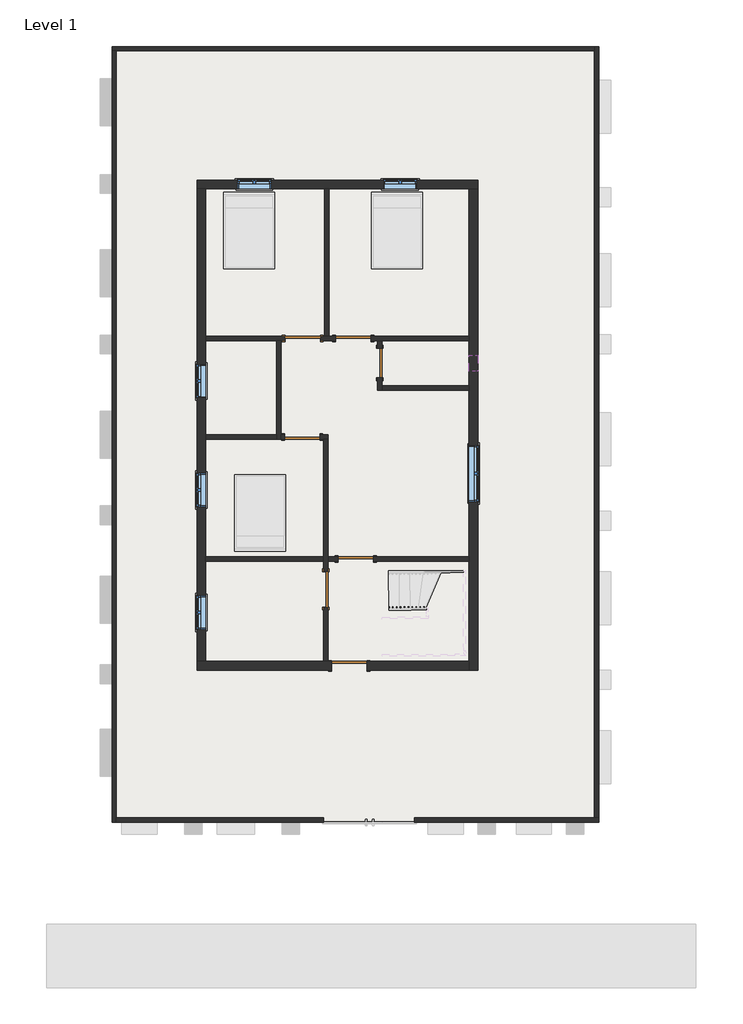
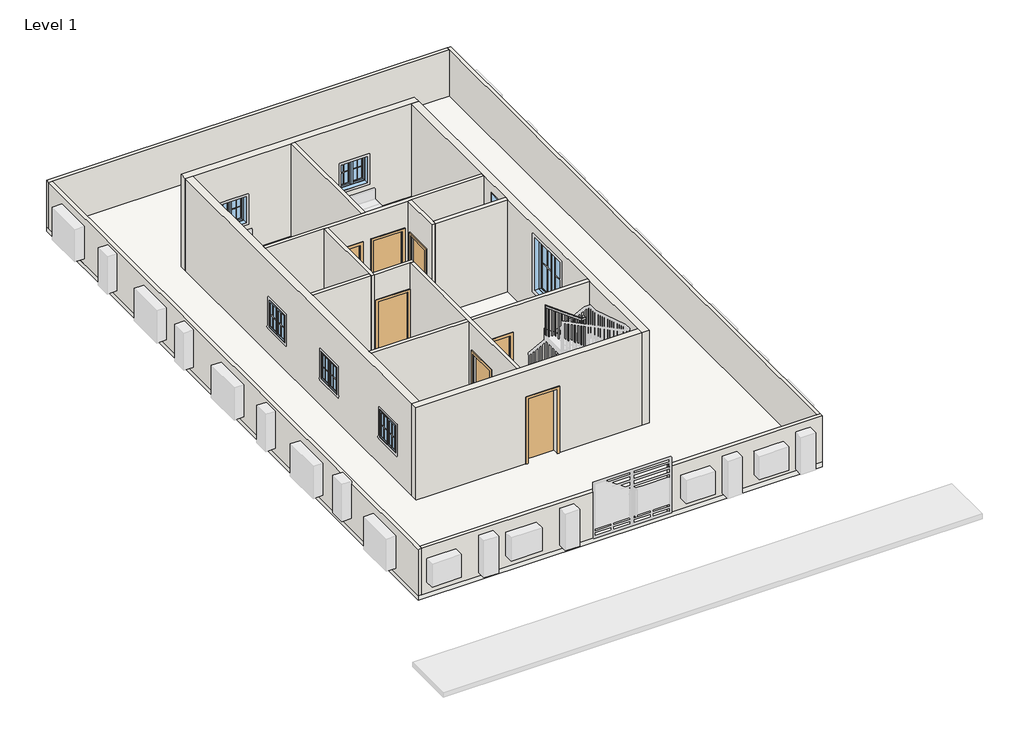
# One storey, part 1 of 2: 18 walls, 7 doors, 7 windows, 1 railing, 1 slab.
"""IFC4 building model written with IfcOpenShell, lengths in millimetres."""

from ifc_helpers import new_model, si_unit, frame, origin, origin_with_axes, place, context, project, spatial, polyline, outline, extrude, faceted_brep, transform, mapped, element, save
from components import door_f2b275c1, door_e5f9f3c4, door_305aa2a5, door_a90ba1ad, window_aa618e30, window_339605e1, window_9ac97e1a

model = new_model("IFC4")

# Units and contexts
model_context = context("Model", 3, world=origin())
ifc_project = project(units=[si_unit("LENGTHUNIT", "METRE", prefix="MILLI")], contexts=[model_context])

# Site, building, storey
site = spatial("IfcSite", under=ifc_project)
building = spatial("IfcBuilding", under=site)
storey = spatial("IfcBuildingStorey", under=building, Name="Level 1", Elevation=0.0)

# Doors
placement = place(None, origin())
door_shape = door_f2b275c1(model_context)
element("IfcDoor", 1, ObjectType="Single-Flush : 30\" x 80\"", at=placement, inside=storey, context=model_context, shape_type="MappedRepresentation", body=[
    mapped(door_shape, transform((-163.0415084, 2144.7435985, 0.0), x_axis=(0.0, 1.0, 0.0), y_axis=(-1.0, 0.0, 0.0), z_axis=(0.0, 0.0, 1.0))),
])
door_2_shape = door_e5f9f3c4(model_context)
element("IfcDoor", 2, ObjectType="Single-Flush : 36\" x 84\"", at=placement, inside=storey, context=model_context, shape_type="MappedRepresentation", body=[
    mapped(door_2_shape, transform((-2156.9415084, 2786.0935985, 0.0), x_axis=(1.0, 0.0, 0.0), y_axis=(0.0, 1.0, 0.0), z_axis=(0.0, 0.0, 1.0))),
])
door_3_shape = door_305aa2a5(model_context)
element("IfcDoor", 3, ObjectType="Single-Flush : 36\" x 84\"", at=placement, inside=storey, context=model_context, shape_type="MappedRepresentation", body=[
    mapped(door_3_shape, transform((-848.8415084, 2786.0935985, 0.0), x_axis=(-1.0, 0.0, 0.0), y_axis=(0.0, -1.0, 0.0), z_axis=(0.0, 0.0, 1.0))),
])
element("IfcDoor", 4, ObjectType="Single-Flush : 36\" x 84\"", at=placement, inside=storey, context=model_context, shape_type="MappedRepresentation", body=[
    mapped(door_3_shape, transform((-2170.1582019, 233.3935985, 0.0), x_axis=(1.0, 0.0, 0.0), y_axis=(0.0, 1.0, 0.0), z_axis=(0.0, 0.0, 1.0))),
])
element("IfcDoor", 5, ObjectType="Single-Flush : 36\" x 84\"", at=placement, inside=storey, context=model_context, shape_type="MappedRepresentation", body=[
    mapped(door_3_shape, transform((-778.9915084, -2928.9064015, 0.0), x_axis=(-1.0, 0.0, 0.0), y_axis=(0.0, -1.0, 0.0), z_axis=(0.0, 0.0, 1.0))),
])
element("IfcDoor", 6, ObjectType="Single-Flush : 36\" x 84\"", at=placement, inside=storey, context=model_context, shape_type="MappedRepresentation", body=[
    mapped(door_3_shape, transform((-1561.0748955, -3709.9564015, 0.0), x_axis=(0.0, 1.0, 0.0), y_axis=(-1.0, 0.0, 0.0), z_axis=(0.0, 0.0, 1.0))),
])
door_4_shape = door_a90ba1ad(model_context)
element("IfcDoor", 7, ObjectType="Single-Flush : 36\" x 84\"", at=placement, inside=storey, context=model_context, shape_type="MappedRepresentation", body=[
    mapped(door_4_shape, transform((-951.4748955, -5691.1564015, 0.0), x_axis=(-1.0, 0.0, 0.0), y_axis=(0.0, -1.0, 0.0), z_axis=(0.0, 0.0, 1.0))),
])

# Railing
element("IfcRailing", 8, ObjectType="Handrail - Rectangular", at=placement, inside=storey, context=model_context, shape_type="SolidModel", body=[
    faceted_brep([(73.2591805, -4146.3303197, 1591.7333333), (73.2591805, -4146.3303197, 1525.1495342), (73.5214139, -4197.1296428, 1525.1495342), (73.5214139, -4197.1296428, 1591.7333333), (1064.2769136, -4141.2145447, 2431.4511215), (1082.90463, -4141.1183857, 2380.6511215), (1083.1668634, -4191.9177089, 2380.6511215), (1064.5391469, -4192.0138678, 2431.4511215), (1144.655904, -4140.7996168, 2431.4511215), (1144.9181373, -4191.59894, 2431.4511215), (1144.9181373, -4191.59894, 2380.6511215), (1144.655904, -4140.7996168, 2380.6511215)], [[[0, 1, 2, 3]], [[1, 0, 4, 5]], [[2, 1, 5, 6]], [[3, 2, 6, 7]], [[0, 3, 7, 4]], [[8, 9, 10, 11]], [[5, 4, 8, 11]], [[6, 5, 11, 10]], [[7, 6, 10, 9]], [[4, 7, 9, 8]]]),
    faceted_brep([(1144.9181373, -4191.59894, 2439.9305642), (1144.9181373, -4191.59894, 2318.648826), (1094.1188142, -4191.8611734, 2318.648826), (1094.1188142, -4191.8611734, 2439.9305642), (1145.9670708, -4394.7962326, 2880.4506209), (1146.2293041, -4445.5955558, 2869.2988968), (1095.429981, -4445.8577892, 2869.2988968), (1095.1677476, -4395.058466, 2880.4506209), (1145.9670708, -4394.7962326, 3131.0424257), (1146.2293041, -4445.5955558, 3080.2424257), (1095.429981, -4445.8577892, 3080.2424257), (1095.1677476, -4395.058466, 3131.0424257), (1146.6226542, -4521.7945406, 3131.0424257), (1146.6226542, -4521.7945406, 3080.2424257), (1095.5610976, -4471.2574507, 3080.2424257), (1095.5610976, -4471.2574507, 3131.0424257), (1019.6243463, -4522.4501239, 3131.0424257), (1002.8333893, -4522.5368013, 3080.2424257), (1002.5711559, -4471.7374781, 3080.2424257), (1019.3621129, -4471.6508008, 3131.0424257), (-100.5579777, -4528.232665, 3962.4), (-100.8202111, -4477.4333418, 3962.4), (-100.8202111, -4477.4333418, 3899.1383775), (-100.5579777, -4528.232665, 3899.1383775)], [[[0, 1, 2, 3]], [[1, 0, 4, 5]], [[2, 1, 5, 6]], [[3, 2, 6, 7]], [[0, 3, 7, 4]], [[5, 4, 8, 9]], [[6, 5, 9, 10]], [[7, 6, 10, 11]], [[4, 7, 11, 8]], [[9, 8, 12, 13]], [[10, 9, 13, 14]], [[11, 10, 14, 15]], [[8, 11, 15, 12]], [[13, 12, 16, 17]], [[14, 13, 17, 18]], [[15, 14, 18, 19]], [[12, 15, 19, 16]], [[20, 21, 22, 23]], [[17, 16, 20, 23]], [[18, 17, 23, 22]], [[19, 18, 22, 21]], [[16, 19, 21, 20]]]),
    extrude(outline(polyline([(235.6690058, -19.05), (221.5309941, 0.0), (1247.144155, 0.0), (1247.144155, -19.05), (235.6690058, -19.05)])), frame((-107.5675843, -4512.3936381, 4125.8108217), z_axis=(-0.005162073969672187, 0.9999866764074069, 0.0), x_axis=(0.0, 0.0, -1.0)), (0.0, 0.0, 1.0), 19.05),
    extrude(outline(polyline([(235.6690059, -19.05), (221.5309942, 0.0), (1171.7414261, 0.0), (1171.7414261, -19.05), (235.6690059, -19.05)])), frame((-5.968938, -4511.8691714, 4050.4080928), z_axis=(-0.005162073969672187, 0.9999866764074069, 0.0), x_axis=(0.0, 0.0, -1.0)), (0.0, 0.0, 1.0), 19.05),
    extrude(outline(polyline([(235.6690058, -19.05), (221.5309941, 0.0), (1096.3386971, 0.0), (1096.3386971, -19.05), (235.6690058, -19.05)])), frame((95.6297083, -4511.3447046, 3975.0053638), z_axis=(-0.005162073969672187, 0.9999866764074069, 0.0), x_axis=(0.0, 0.0, -1.0)), (0.0, 0.0, 1.0), 19.05),
    extrude(outline(polyline([(235.6690059, -19.0499999), (221.5309942, 0.0), (1190.2693016, 0.0), (1190.2693016, -19.0499999), (235.6690059, -19.0499999)])), frame((197.2283547, -4510.8202379, 3899.6026349), z_axis=(-0.005162073969672187, 0.9999866764074069, 0.0), x_axis=(0.0, 0.0, -1.0)), (0.0, 0.0, 1.0), 19.05),
    extrude(outline(polyline([(235.6690058, -19.05), (221.5309942, 0.0), (1114.8665726, 0.0), (1114.8665726, -19.05), (235.6690058, -19.05)])), frame((298.827001, -4510.2957712, 3824.1999059), z_axis=(-0.005162073969672187, 0.9999866764074069, 0.0), x_axis=(0.0, 0.0, -1.0)), (0.0, 0.0, 1.0), 19.05),
    extrude(outline(polyline([(235.6690058, -19.05), (221.5309941, 0.0), (1039.4638436, 0.0), (1039.4638436, -19.05), (235.6690058, -19.05)])), frame((400.4256473, -4509.7713045, 3748.7971769), z_axis=(-0.005162073969672187, 0.9999866764074069, 0.0), x_axis=(0.0, 0.0, -1.0)), (0.0, 0.0, 1.0), 19.05),
    extrude(outline(polyline([(235.6690058, -19.05), (221.5309942, 0.0), (1133.394448, 0.0), (1133.394448, -19.05), (235.6690058, -19.05)])), frame((502.0242936, -4509.2468378, 3673.394448), z_axis=(-0.005162073969672187, 0.9999866764074069, 0.0), x_axis=(0.0, 0.0, -1.0)), (0.0, 0.0, 1.0), 19.05),
    extrude(outline(polyline([(235.6690058, -19.05), (221.5309941, 0.0), (1057.991719, 0.0), (1057.991719, -19.05), (235.6690058, -19.05)])), frame((603.6229399, -4508.7223711, 3597.991719), z_axis=(-0.005162073969672187, 0.9999866764074069, 0.0), x_axis=(0.0, 0.0, -1.0)), (0.0, 0.0, 1.0), 19.05),
    extrude(outline(polyline([(235.6690059, -19.05), (221.5309942, 0.0), (1151.9223234, 0.0), (1151.9223234, -19.05), (235.6690059, -19.05)])), frame((705.2215863, -4508.1979044, 3522.5889901), z_axis=(-0.005162073969672187, 0.9999866764074069, 0.0), x_axis=(0.0, 0.0, -1.0)), (0.0, 0.0, 1.0), 19.05),
    extrude(outline(polyline([(235.6690058, -19.05), (221.5309941, 0.0), (1076.5195944, 0.0), (1076.5195944, -19.05), (235.6690058, -19.05)])), frame((806.8202326, -4507.6734376, 3447.1862611), z_axis=(-0.005162073969672187, 0.9999866764074069, 0.0), x_axis=(0.0, 0.0, -1.0)), (0.0, 0.0, 1.0), 19.05),
    extrude(outline(polyline([(235.6690059, -19.05), (221.5309942, 0.0), (1170.4501989, 0.0), (1170.4501989, -19.05), (235.6690059, -19.05)])), frame((908.4188789, -4507.1489709, 3371.7835322), z_axis=(-0.005162073969672187, 0.9999866764074069, 0.0), x_axis=(0.0, 0.0, -1.0)), (0.0, 0.0, 1.0), 19.05),
    extrude(outline(polyline([(235.6690058, -19.05), (221.5309942, 0.0), (1095.0474699, 0.0), (1095.0474699, -19.05), (235.6690058, -19.05)])), frame((1010.0175252, -4506.6245042, 3296.3808032), z_axis=(-0.005162073969672187, 0.9999866764074069, 0.0), x_axis=(0.0, 0.0, -1.0)), (0.0, 0.0, 1.0), 19.05),
    extrude(outline(polyline([(1111.3867174, -4461.6506297), (1130.4364636, -4461.5522922), (1130.5348011, -4480.6020384), (1111.4850549, -4480.7003759), (1111.3867174, -4461.6506297)])), frame((0.0, 0.0, 2032.0), z_axis=(0.0, 0.0, 1.0), x_axis=(1.0, 0.0, 0.0)), (0.0, 0.0, 1.0), 1048.2424257),
    extrude(outline(polyline([(207.9506224, -19.05), (249.2493777, 0.0), (1070.0372089, 0.0), (1070.0372089, -19.05), (207.9506224, -19.05)])), frame((1110.8622507, -4360.0519834, 2932.7038756), z_axis=(0.9999866764074068, 0.005162073969671281, 0.0), x_axis=(0.0, 0.0, -1.0)), (0.0, 0.0, 1.0), 19.05),
    extrude(outline(polyline([(207.9506224, -19.05), (249.2493777, 0.0), (1019.110514, 0.0), (1019.110514, -19.05), (207.9506224, -19.05)])), frame((1110.3377839, -4258.4533371, 2712.4438473), z_axis=(0.9999866764074068, 0.005162073969671281, 0.0), x_axis=(0.0, 0.0, -1.0)), (0.0, 0.0, 1.0), 19.05),
    extrude(outline(polyline([(1079.9010561, -4176.0593559), (1079.8027186, -4157.0096098), (1098.8524648, -4156.9112722), (1098.9508023, -4175.9610184), (1079.9010561, -4176.0593559)])), frame((0.0, 0.0, 1354.6666667), z_axis=(0.0, 0.0, 1.0), x_axis=(1.0, 0.0, 0.0)), (0.0, 0.0, 1.0), 1025.9844548),
    extrude(outline(polyline([(220.5293015, -19.05), (236.6706986, 0.0), (1343.2032603, 0.0), (1343.2032603, -19.05), (220.5293015, -19.05)])), frame((978.3024098, -4176.5838227, 2528.5365936), z_axis=(-0.005162073969671482, 0.9999866764074068, 0.0), x_axis=(0.0, 0.0, -1.0)), (0.0, 0.0, 1.0), 19.05),
    extrude(outline(polyline([(220.5293015, -19.05), (236.6706985, 0.0), (1257.1158092, 0.0), (1257.1158092, -19.05), (220.5293015, -19.05)])), frame((876.7037635, -4177.1082894, 2442.4491425), z_axis=(-0.005162073969671482, 0.9999866764074068, 0.0), x_axis=(0.0, 0.0, -1.0)), (0.0, 0.0, 1.0), 19.05),
    extrude(outline(polyline([(220.5293015, -19.05), (236.6706986, 0.0), (1340.3616915, 0.0), (1340.3616915, -19.05), (220.5293015, -19.05)])), frame((775.1051171, -4177.6327561, 2356.3616915), z_axis=(-0.005162073969671482, 0.9999866764074068, 0.0), x_axis=(0.0, 0.0, -1.0)), (0.0, 0.0, 1.0), 19.05),
    extrude(outline(polyline([(220.5293014, -19.05), (236.6706985, 0.0), (1254.2742404, 0.0), (1254.2742404, -19.05), (220.5293014, -19.05)])), frame((673.5064708, -4178.1572228, 2270.2742404), z_axis=(-0.005162073969671482, 0.9999866764074068, 0.0), x_axis=(0.0, 0.0, -1.0)), (0.0, 0.0, 1.0), 19.05),
    extrude(outline(polyline([(220.5293015, -19.05), (236.6706985, 0.0), (1337.5201227, 0.0), (1337.5201227, -19.05), (220.5293015, -19.05)])), frame((571.9078245, -4178.6816895, 2184.1867894), z_axis=(-0.005162073969671482, 0.9999866764074068, 0.0), x_axis=(0.0, 0.0, -1.0)), (0.0, 0.0, 1.0), 19.05),
    extrude(outline(polyline([(220.5293015, -19.05), (236.6706986, 0.0), (1251.4326717, 0.0), (1251.4326717, -19.05), (220.5293015, -19.05)])), frame((470.3091782, -4179.2061562, 2098.0993384), z_axis=(-0.005162073969671482, 0.9999866764074068, 0.0), x_axis=(0.0, 0.0, -1.0)), (0.0, 0.0, 1.0), 19.05),
    extrude(outline(polyline([(220.5293014, -19.0499999), (236.6706985, 0.0), (1165.3452206, 0.0), (1165.3452206, -19.0499999), (220.5293014, -19.0499999)])), frame((368.7105319, -4179.7306229, 2012.0118873), z_axis=(-0.005162073969671482, 0.9999866764074068, 0.0), x_axis=(0.0, 0.0, -1.0)), (0.0, 0.0, 1.0), 19.05),
    extrude(outline(polyline([(220.5293015, -19.05), (236.6706986, 0.0), (1248.591103, 0.0), (1248.591103, -19.05), (220.5293015, -19.05)])), frame((267.1118855, -4180.2550897, 1925.9244363), z_axis=(-0.005162073969671482, 0.9999866764074068, 0.0), x_axis=(0.0, 0.0, -1.0)), (0.0, 0.0, 1.0), 19.05),
    extrude(outline(polyline([(220.5293014, -19.05), (236.6706985, 0.0), (1162.5036519, 0.0), (1162.5036519, -19.05), (220.5293014, -19.05)])), frame((165.5132392, -4180.7795564, 1839.8369852), z_axis=(-0.005162073969671482, 0.9999866764074068, 0.0), x_axis=(0.0, 0.0, -1.0)), (0.0, 0.0, 1.0), 19.05),
    extrude(outline(polyline([(1111.5178341, -4487.0502913), (1130.5675802, -4486.9519538), (1130.6659177, -4506.0017), (1111.6161716, -4506.1000375), (1111.5178341, -4487.0502913)])), frame((0.0, 0.0, 2032.0), z_axis=(0.0, 0.0, 1.0), x_axis=(1.0, 0.0, 0.0)), (0.0, 0.0, 1.0), 1048.2424257),
    extrude(outline(polyline([(1109.9116547, -4175.9044369), (1109.8133172, -4156.8546908), (1128.8630634, -4156.7563533), (1128.9614009, -4175.8060994), (1109.9116547, -4175.9044369)])), frame((0.0, 0.0, 1524.0), z_axis=(0.0, 0.0, 1.0), x_axis=(1.0, 0.0, 0.0)), (0.0, 0.0, 1.0), 856.6511215),
    extrude(outline(polyline([(235.6690058, -19.05), (221.5309941, 0.0), (1242.0027049, 0.0), (1242.0027049, -19.05), (235.6690058, -19.05)])), frame((-100.6399256, -4512.3578765, 4120.6693716), z_axis=(-0.005162073969672187, 0.9999866764074069, 0.0), x_axis=(0.0, 0.0, -1.0)), (0.0, 0.0, 1.0), 19.05),
    extrude(outline(polyline([(220.5293014, -19.05), (236.6706985, 0.0), (1084.4868994, 0.0), (1084.4868994, -19.05), (220.5293014, -19.05)])), frame((73.439466, -4181.2548543, 1761.8202327), z_axis=(-0.005162073969671482, 0.9999866764074068, 0.0), x_axis=(0.0, 0.0, -1.0)), (0.0, 0.0, 1.0), 19.05),
])

# Slab
element("IfcSlab", 9, ObjectType="Generic - 12\"", at=placement, inside=storey, context=model_context, shape_type="SweptSolid", body=[
    extrude(outline(polyline([(5515.9206788, 10339.756004), (5515.9206788, -9738.943996), (-7095.1793212, -9738.943996), (-7095.1793212, 10339.756004), (5515.9206788, 10339.756004)])), frame((0.0, 0.0, -152.4), z_axis=(0.0, 0.0, 1.0), x_axis=(1.0, 0.0, 0.0)), (0.0, 0.0, 1.0), 152.4),
])

# Walls
element("IfcWall", 10, ObjectType="WALL4.5\"", at=placement, inside=storey, context=model_context, shape_type="Brep", body=[
    faceted_brep([(-1699.7415084, 2728.9435985, 0.0), (-1306.0415084, 2728.9435985, 0.0), (-1306.0415084, 2728.9435985, 2133.6), (-391.6415084, 2728.9435985, 2133.6), (-391.6415084, 2728.9435985, 0.0), (-220.1915084, 2728.9435985, 0.0), (-105.8915084, 2728.9435985, 0.0), (2154.7084916, 2728.9435985, 0.0), (2154.7084916, 2728.9435985, 3048.0), (-105.8915084, 2728.9435985, 3048.0), (-220.1915084, 2728.9435985, 3048.0), (-2722.0915084, 2728.9435985, 3048.0), (-2836.3915084, 2728.9435985, 3048.0), (-4665.1915084, 2728.9435985, 3048.0), (-4665.1915084, 2728.9435985, 0.0), (-2836.3915084, 2728.9435985, 0.0), (-2722.0915084, 2728.9435985, 0.0), (-2614.1415084, 2728.9435985, 0.0), (-2614.1415084, 2728.9435985, 2133.6), (-1699.7415084, 2728.9435985, 2133.6), (-1306.0415084, 2843.2435985, 2133.6), (-1306.0415084, 2843.2435985, 0.0), (-1477.4915084, 2843.2435985, 0.0), (-1591.7915084, 2843.2435985, 0.0), (-1699.7415084, 2843.2435985, 0.0), (-1699.7415084, 2843.2435985, 2133.6), (-2614.1415084, 2843.2435985, 2133.6), (-2614.1415084, 2843.2435985, 0.0), (-4665.1915084, 2843.2435985, 0.0), (-4665.1915084, 2843.2435985, 3048.0), (-1591.7915084, 2843.2435985, 3048.0), (-1477.4915084, 2843.2435985, 3048.0), (2154.7084916, 2843.2435985, 3048.0), (2154.7084916, 2843.2435985, 0.0), (-391.6415084, 2843.2435985, 0.0), (-391.6415084, 2843.2435985, 2133.6)], [[[0, 1, 2, 3, 4, 5, 6, 7, 8, 9, 10, 11, 12, 13, 14, 15, 16, 17, 18, 19]], [[20, 21, 22, 23, 24, 25, 26, 27, 28, 29, 30, 31, 32, 33, 34, 35]], [[17, 16, 15, 14, 28, 27]], [[34, 33, 7, 6, 5, 4]], [[24, 23, 22, 21, 1, 0]], [[8, 7, 33, 32]], [[14, 13, 29, 28]], [[25, 24, 0, 19]], [[26, 25, 19, 18]], [[27, 26, 18, 17]], [[2, 1, 21, 20]], [[3, 2, 20, 35]], [[4, 3, 35, 34]], [[13, 12, 11, 10, 9, 8, 32, 31, 30, 29]]]),
])
element("IfcWall", 11, ObjectType="WALL4.5\"", at=placement, inside=storey, context=model_context, shape_type="SweptSolid", body=[
    extrude(outline(polyline([(-1591.7915084, 2843.2435985), (-1591.7915084, 6653.2435985), (-1477.4915084, 6653.2435985), (-1477.4915084, 2843.2435985), (-1591.7915084, 2843.2435985)])), origin_with_axes(), (0.0, 0.0, 1.0), 3048.0),
])
element("IfcWall", 12, ObjectType="WALL4.5\"", at=placement, inside=storey, context=model_context, shape_type="Brep", body=[
    faceted_brep([(-2836.3915084, 2728.9435985, 0.0), (-2836.3915084, 290.5435985, 0.0), (-2836.3915084, 176.2435985, 0.0), (-2836.3915084, 176.2435985, 3048.0), (-2836.3915084, 290.5435985, 3048.0), (-2836.3915084, 2728.9435985, 3048.0), (-2722.0915084, 2728.9435985, 0.0), (-2722.0915084, 2728.9435985, 3048.0), (-2722.0915084, 290.5435985, 3048.0), (-2722.0915084, 176.2435985, 3048.0), (-2722.0915084, 176.2435985, 0.0), (-2722.0915084, 290.5435985, 0.0)], [[[0, 1, 2, 3, 4, 5]], [[6, 7, 8, 9, 10, 11]], [[2, 1, 0, 6, 11, 10]], [[0, 5, 7, 6]], [[3, 2, 10, 9]], [[5, 4, 3, 9, 8, 7]]]),
])
element("IfcWall", 13, ObjectType="WALL4.5\"", at=placement, inside=storey, context=model_context, shape_type="SweptSolid", body=[
    extrude(outline(polyline([(-2836.3915084, 176.2435985), (-4665.1915084, 176.2435985), (-4665.1915084, 290.5435985), (-2836.3915084, 290.5435985), (-2836.3915084, 176.2435985)])), origin_with_axes(), (0.0, 0.0, 1.0), 3048.0),
])
element("IfcWall", 14, ObjectType="WALL4.5\"", at=placement, inside=storey, context=model_context, shape_type="Brep", body=[
    faceted_brep([(-1712.9582019, 176.2435985, 2133.6), (-1712.9582019, 176.2435985, 0.0), (-1618.2248955, 176.2435985, 0.0), (-1503.9248955, 176.2435985, 0.0), (-1502.8915084, 176.2435985, 0.0), (-1502.8915084, 176.2435985, 3048.0), (-1503.9248955, 176.2435985, 3048.0), (-1618.2248955, 176.2435985, 3048.0), (-2722.0915084, 176.2435985, 3048.0), (-2722.0915084, 176.2435985, 0.0), (-2627.3582019, 176.2435985, 0.0), (-2627.3582019, 176.2435985, 2133.6), (-1502.8915084, 290.5435985, 0.0), (-1712.9582019, 290.5435985, 0.0), (-1712.9582019, 290.5435985, 2133.6), (-2627.3582019, 290.5435985, 2133.6), (-2627.3582019, 290.5435985, 0.0), (-2722.0915084, 290.5435985, 0.0), (-2722.0915084, 290.5435985, 3048.0), (-1502.8915084, 290.5435985, 3048.0)], [[[0, 1, 2, 3, 4, 5, 6, 7, 8, 9, 10, 11]], [[12, 13, 14, 15, 16, 17, 18, 19]], [[10, 9, 17, 16]], [[4, 3, 2, 1, 13, 12]], [[5, 4, 12, 19]], [[9, 8, 18, 17]], [[14, 13, 1, 0]], [[15, 14, 0, 11]], [[16, 15, 11, 10]], [[8, 7, 6, 5, 19, 18]]]),
])
element("IfcWall", 15, ObjectType="WALL4.5\"", at=placement, inside=storey, context=model_context, shape_type="Brep", body=[
    faceted_brep([(-1618.2248955, 176.2435985, 0.0), (-1618.2248955, -2871.7564015, 0.0), (-1618.2248955, -2986.0564015, 0.0), (-1618.2248955, -3252.7564015, 0.0), (-1618.2248955, -3252.7564015, 2133.6), (-1618.2248955, -4167.1564015, 2133.6), (-1618.2248955, -4167.1564015, 0.0), (-1618.2248955, -5576.8564015, 0.0), (-1618.2248955, -5576.8564015, 3048.0), (-1618.2248955, -2986.0564015, 3048.0), (-1618.2248955, -2871.7564015, 3048.0), (-1618.2248955, 176.2435985, 3048.0), (-1503.9248955, -3252.7564015, 2133.6), (-1503.9248955, -3252.7564015, 0.0), (-1503.9248955, -2986.0564015, 0.0), (-1503.9248955, -2871.7564015, 0.0), (-1503.9248955, 176.2435985, 0.0), (-1503.9248955, 176.2435985, 3048.0), (-1503.9248955, -2871.7564015, 3048.0), (-1503.9248955, -2986.0564015, 3048.0), (-1503.9248955, -5576.8564015, 3048.0), (-1503.9248955, -5576.8564015, 0.0), (-1503.9248955, -4167.1564015, 0.0), (-1503.9248955, -4167.1564015, 2133.6)], [[[0, 1, 2, 3, 4, 5, 6, 7, 8, 9, 10, 11]], [[12, 13, 14, 15, 16, 17, 18, 19, 20, 21, 22, 23]], [[22, 21, 7, 6]], [[16, 15, 14, 13, 3, 2, 1, 0]], [[8, 7, 21, 20]], [[0, 11, 17, 16]], [[4, 3, 13, 12]], [[5, 4, 12, 23]], [[6, 5, 23, 22]], [[11, 10, 9, 8, 20, 19, 18, 17]]]),
])
element("IfcWall", 16, ObjectType="WALL4.5\"", at=placement, inside=storey, context=model_context, shape_type="SweptSolid", body=[
    extrude(outline(polyline([(0.0, 2154.7084916), (3048.0, 2154.7084916), (3048.0, -1503.9248955), (0.0, -1503.9248955), (0.0, -1236.1915084), (2133.6, -1236.1915084), (2133.6, -321.7915084), (0.0, -321.7915084), (0.0, 2154.7084916)])), frame((0.0, -2986.0564015, 0.0), z_axis=(0.0, 1.0, 0.0), x_axis=(0.0, 0.0, 1.0)), (0.0, 0.0, 1.0), 114.3),
    extrude(outline(polyline([(-4665.1915084, -2986.0564015), (-4665.1915084, -2871.7564015), (-1618.2248955, -2871.7564015), (-1618.2248955, -2986.0564015), (-4665.1915084, -2986.0564015)])), origin_with_axes(), (0.0, 0.0, 1.0), 3048.0),
])
element("IfcWall", 17, ObjectType="WALL4.5\"", at=placement, inside=storey, context=model_context, shape_type="Brep", body=[
    faceted_brep([(-220.1915084, 2728.9435985, 0.0), (-220.1915084, 2525.7435985, 0.0), (-220.1915084, 2525.7435985, 2032.0), (-220.1915084, 1763.7435985, 2032.0), (-220.1915084, 1763.7435985, 0.0), (-220.1915084, 1446.2435985, 0.0), (-220.1915084, 1446.2435985, 3048.0), (-220.1915084, 2728.9435985, 3048.0), (-105.8915084, 2525.7435985, 2032.0), (-105.8915084, 2525.7435985, 0.0), (-105.8915084, 2728.9435985, 0.0), (-105.8915084, 2728.9435985, 3048.0), (-105.8915084, 1560.5435985, 3048.0), (-105.8915084, 1446.2435985, 3048.0), (-105.8915084, 1446.2435985, 0.0), (-105.8915084, 1560.5435985, 0.0), (-105.8915084, 1763.7435985, 0.0), (-105.8915084, 1763.7435985, 2032.0)], [[[0, 1, 2, 3, 4, 5, 6, 7]], [[8, 9, 10, 11, 12, 13, 14, 15, 16, 17]], [[10, 9, 1, 0]], [[16, 15, 14, 5, 4]], [[0, 7, 11, 10]], [[6, 5, 14, 13]], [[2, 1, 9, 8]], [[3, 2, 8, 17]], [[4, 3, 17, 16]], [[7, 6, 13, 12, 11]]]),
])
element("IfcWall", 18, ObjectType="WALL4.5\"", at=placement, inside=storey, context=model_context, shape_type="SweptSolid", body=[
    extrude(outline(polyline([(2154.7084916, 1446.2435985), (-105.8915084, 1446.2435985), (-105.8915084, 1560.5435985), (2154.7084916, 1560.5435985), (2154.7084916, 1446.2435985)])), origin_with_axes(), (0.0, 0.0, 1.0), 3048.0),
])
element("IfcWall", 19, ObjectType="WALL4.5\"", at=placement, inside=storey, context=model_context, shape_type="Brep", body=[
    faceted_brep([(-7095.1793212, 10225.456004, 0.0), (-6980.8793212, 10225.456004, 0.0), (5401.6206788, 10225.456004, 0.0), (5401.6206788, 10225.456004, 1524.0), (-6980.8793212, 10225.456004, 1524.0), (-7095.1793212, 10225.456004, 1524.0), (-7095.1793212, 10339.756004, 0.0), (-7095.1793212, 10339.756004, 1524.0), (5401.6206788, 10339.756004, 1524.0), (5401.6206788, 10339.756004, 0.0)], [[[0, 1, 2, 3, 4, 5]], [[6, 7, 8, 9]], [[2, 1, 0, 6, 9]], [[5, 4, 3, 8, 7]], [[0, 5, 7, 6]], [[3, 2, 9, 8]]]),
])
element("IfcWall", 20, ObjectType="WALL4.5\"", at=placement, inside=storey, context=model_context, shape_type="Brep", body=[
    faceted_brep([(-6980.8793212, -9738.943996, 0.0), (-6980.8793212, -9624.643996, 0.0), (-6980.8793212, 10225.456004, 0.0), (-6980.8793212, 10225.456004, 1524.0), (-6980.8793212, -9624.643996, 1524.0), (-6980.8793212, -9738.943996, 1524.0), (-7095.1793212, -9738.943996, 0.0), (-7095.1793212, -9738.943996, 1524.0), (-7095.1793212, 10225.456004, 1524.0), (-7095.1793212, 10225.456004, 0.0)], [[[0, 1, 2, 3, 4, 5]], [[6, 7, 8, 9]], [[2, 1, 0, 6, 9]], [[5, 4, 3, 8, 7]], [[0, 5, 7, 6]], [[3, 2, 9, 8]]]),
])
element("IfcWall", 21, ObjectType="WALL4.5\"", at=placement, inside=storey, context=model_context, shape_type="Brep", body=[
    faceted_brep([(5515.9206788, -9624.643996, 0.0), (5401.6206788, -9624.643996, 0.0), (734.3706788, -9624.643996, 0.0), (734.3706788, -9624.643996, 1524.0), (5401.6206788, -9624.643996, 1524.0), (5515.9206788, -9624.643996, 1524.0), (5515.9206788, -9738.943996, 0.0), (5515.9206788, -9738.943996, 1524.0), (734.3706788, -9738.943996, 1524.0), (734.3706788, -9738.943996, 0.0)], [[[0, 1, 2, 3, 4, 5]], [[6, 7, 8, 9]], [[2, 1, 0, 6, 9]], [[3, 2, 9, 8]], [[5, 4, 3, 8, 7]], [[0, 5, 7, 6]]]),
])
element("IfcWall", 22, ObjectType="WALL4.5\"", at=placement, inside=storey, context=model_context, shape_type="Brep", body=[
    faceted_brep([(5401.6206788, 10339.756004, 0.0), (5401.6206788, 10225.456004, 0.0), (5401.6206788, -9624.643996, 0.0), (5401.6206788, -9624.643996, 1524.0), (5401.6206788, 10225.456004, 1524.0), (5401.6206788, 10339.756004, 1524.0), (5515.9206788, 10339.756004, 0.0), (5515.9206788, 10339.756004, 1524.0), (5515.9206788, -9624.643996, 1524.0), (5515.9206788, -9624.643996, 0.0)], [[[0, 1, 2, 3, 4, 5]], [[6, 7, 8, 9]], [[2, 1, 0, 6, 9]], [[5, 4, 3, 8, 7]], [[0, 5, 7, 6]], [[3, 2, 9, 8]]]),
])
element("IfcWall", 23, ObjectType="WALL4.5\"", at=placement, inside=storey, context=model_context, shape_type="SweptSolid", body=[
    extrude(outline(polyline([(-6980.8793212, -9624.643996), (-1618.2248955, -9624.643996), (-1618.2248955, -9738.943996), (-6980.8793212, -9738.943996), (-6980.8793212, -9624.643996)])), origin_with_axes(), (0.0, 0.0, 1.0), 1524.0),
])
element("IfcWall", 24, ObjectType="WALL9\"", at=placement, inside=storey, context=model_context, shape_type="Brep", body=[
    faceted_brep([(-4893.7915084, 6653.2435985, 0.0), (-4665.1915084, 6653.2435985, 0.0), (-1591.7915084, 6653.2435985, 0.0), (-1477.4915084, 6653.2435985, 0.0), (2154.7084916, 6653.2435985, 0.0), (2383.3084916, 6653.2435985, 0.0), (2383.3084916, 6653.2435985, 3048.0), (2154.7084916, 6653.2435985, 3048.0), (-1477.4915084, 6653.2435985, 3048.0), (-1591.7915084, 6653.2435985, 3048.0), (-4665.1915084, 6653.2435985, 3048.0), (-4893.7915084, 6653.2435985, 3048.0), (-2976.0915084, 6653.2435985, 1828.8), (-2976.0915084, 6653.2435985, 914.4), (-3839.6915084, 6653.2435985, 914.4), (-3839.6915084, 6653.2435985, 1828.8), (798.9834916, 6653.2435985, 1828.8), (798.9834916, 6653.2435985, 914.4), (-64.6165084, 6653.2435985, 914.4), (-64.6165084, 6653.2435985, 1828.8), (-4893.7915084, 6881.8435985, 0.0), (-4893.7915084, 6881.8435985, 3048.0), (2383.3084916, 6881.8435985, 3048.0), (2383.3084916, 6881.8435985, 0.0), (-2976.0915084, 6881.8435985, 1828.8), (-3839.6915084, 6881.8435985, 1828.8), (-3839.6915084, 6881.8435985, 914.4), (-2976.0915084, 6881.8435985, 914.4), (798.9834916, 6881.8435985, 1828.8), (-64.6165084, 6881.8435985, 1828.8), (-64.6165084, 6881.8435985, 914.4), (798.9834916, 6881.8435985, 914.4)], [[[0, 1, 2, 3, 4, 5, 6, 7, 8, 9, 10, 11], [12, 13, 14, 15], [16, 17, 18, 19]], [[20, 21, 22, 23], [24, 25, 26, 27], [28, 29, 30, 31]], [[5, 4, 3, 2, 1, 0, 20, 23]], [[6, 5, 23, 22]], [[0, 11, 21, 20]], [[13, 12, 24, 27]], [[14, 13, 27, 26]], [[15, 14, 26, 25]], [[12, 15, 25, 24]], [[17, 16, 28, 31]], [[18, 17, 31, 30]], [[19, 18, 30, 29]], [[16, 19, 29, 28]], [[11, 10, 9, 8, 7, 6, 22, 21]]]),
])
element("IfcWall", 25, ObjectType="WALL9\"", at=placement, inside=storey, context=model_context, shape_type="Brep", body=[
    faceted_brep([(2154.7084916, 6653.2435985, 0.0), (2154.7084916, 2843.2435985, 0.0), (2154.7084916, 2728.9435985, 0.0), (2154.7084916, 1560.5435985, 0.0), (2154.7084916, 1446.2435985, 0.0), (2154.7084916, -2871.7564015, 0.0), (2154.7084916, -2986.0564015, 0.0), (2154.7084916, -5576.8564015, 0.0), (2154.7084916, -5805.4564015, 0.0), (2154.7084916, -5805.4564015, 3048.0), (2154.7084916, -5576.8564015, 3048.0), (2154.7084916, -2986.0564015, 3048.0), (2154.7084916, -2871.7564015, 3048.0), (2154.7084916, 1446.2435985, 3048.0), (2154.7084916, 1560.5435985, 3048.0), (2154.7084916, 2728.9435985, 3048.0), (2154.7084916, 2843.2435985, 3048.0), (2154.7084916, 6653.2435985, 3048.0), (2154.7084916, 1941.5435985, 2743.2), (2154.7084916, 1941.5435985, 2133.6), (2154.7084916, 2347.9435985, 2133.6), (2154.7084916, 2347.9435985, 2743.2), (2154.7084916, -1436.6564015, 2743.2), (2154.7084916, -1436.6564015, 914.4), (2154.7084916, 11.1435985, 914.4), (2154.7084916, 11.1435985, 2743.2), (2383.3084916, 6653.2435985, 0.0), (2383.3084916, 6653.2435985, 3048.0), (2383.3084916, -5805.4564015, 3048.0), (2383.3084916, -5805.4564015, 0.0), (2383.3084916, 1941.5435985, 2743.2), (2383.3084916, 2347.9435985, 2743.2), (2383.3084916, 2347.9435985, 2133.6), (2383.3084916, 1941.5435985, 2133.6), (2383.3084916, -1436.6564015, 2743.2), (2383.3084916, 11.1435985, 2743.2), (2383.3084916, 11.1435985, 914.4), (2383.3084916, -1436.6564015, 914.4)], [[[0, 1, 2, 3, 4, 5, 6, 7, 8, 9, 10, 11, 12, 13, 14, 15, 16, 17], [18, 19, 20, 21], [22, 23, 24, 25]], [[26, 27, 28, 29], [30, 31, 32, 33], [34, 35, 36, 37]], [[8, 7, 6, 5, 4, 3, 2, 1, 0, 26, 29]], [[0, 17, 27, 26]], [[9, 8, 29, 28]], [[19, 18, 30, 33]], [[20, 19, 33, 32]], [[21, 20, 32, 31]], [[18, 21, 31, 30]], [[23, 22, 34, 37]], [[24, 23, 37, 36]], [[25, 24, 36, 35]], [[22, 25, 35, 34]], [[17, 16, 15, 14, 13, 12, 11, 10, 9, 28, 27]]]),
])
element("IfcWall", 26, ObjectType="WALL9\"", at=placement, inside=storey, context=model_context, shape_type="Brep", body=[
    faceted_brep([(-1408.6748955, -5576.8564015, 2133.6), (-1408.6748955, -5576.8564015, 0.0), (-1503.9248955, -5576.8564015, 0.0), (-1618.2248955, -5576.8564015, 0.0), (-4665.1915084, -5576.8564015, 0.0), (-4893.7915084, -5576.8564015, 0.0), (-4893.7915084, -5576.8564015, 3048.0), (-4665.1915084, -5576.8564015, 3048.0), (-1618.2248955, -5576.8564015, 3048.0), (-1503.9248955, -5576.8564015, 3048.0), (2154.7084916, -5576.8564015, 3048.0), (2154.7084916, -5576.8564015, 0.0), (-494.2748955, -5576.8564015, 0.0), (-494.2748955, -5576.8564015, 2133.6), (-4893.7915084, -5805.4564015, 0.0), (-1408.6748955, -5805.4564015, 0.0), (-1408.6748955, -5805.4564015, 2133.6), (-494.2748955, -5805.4564015, 2133.6), (-494.2748955, -5805.4564015, 0.0), (2154.7084916, -5805.4564015, 0.0), (2154.7084916, -5805.4564015, 3048.0), (-4893.7915084, -5805.4564015, 3048.0)], [[[0, 1, 2, 3, 4, 5, 6, 7, 8, 9, 10, 11, 12, 13]], [[14, 15, 16, 17, 18, 19, 20, 21]], [[12, 11, 19, 18]], [[5, 4, 3, 2, 1, 15, 14]], [[11, 10, 20, 19]], [[6, 5, 14, 21]], [[16, 15, 1, 0]], [[17, 16, 0, 13]], [[18, 17, 13, 12]], [[10, 9, 8, 7, 6, 21, 20]]]),
])
element("IfcWall", 27, ObjectType="WALL9\"", at=placement, inside=storey, context=model_context, shape_type="Brep", body=[
    faceted_brep([(-4665.1915084, -5576.8564015, 0.0), (-4665.1915084, -2986.0564015, 0.0), (-4665.1915084, -2871.7564015, 0.0), (-4665.1915084, 176.2435985, 0.0), (-4665.1915084, 290.5435985, 0.0), (-4665.1915084, 2728.9435985, 0.0), (-4665.1915084, 2843.2435985, 0.0), (-4665.1915084, 6653.2435985, 0.0), (-4665.1915084, 6653.2435985, 3048.0), (-4665.1915084, 2843.2435985, 3048.0), (-4665.1915084, 2728.9435985, 3048.0), (-4665.1915084, 290.5435985, 3048.0), (-4665.1915084, 176.2435985, 3048.0), (-4665.1915084, -2871.7564015, 3048.0), (-4665.1915084, -2986.0564015, 3048.0), (-4665.1915084, -5576.8564015, 3048.0), (-4665.1915084, 2112.9935985, 1828.8), (-4665.1915084, 2112.9935985, 914.4), (-4665.1915084, 1249.3935985, 914.4), (-4665.1915084, 1249.3935985, 1828.8), (-4665.1915084, -706.4064015, 1828.8), (-4665.1915084, -706.4064015, 914.4), (-4665.1915084, -1570.0064015, 914.4), (-4665.1915084, -1570.0064015, 1828.8), (-4665.1915084, -3878.2314015, 1828.8), (-4665.1915084, -3878.2314015, 914.4), (-4665.1915084, -4741.8314015, 914.4), (-4665.1915084, -4741.8314015, 1828.8), (-4893.7915084, -5576.8564015, 0.0), (-4893.7915084, -5576.8564015, 3048.0), (-4893.7915084, 6653.2435985, 3048.0), (-4893.7915084, 6653.2435985, 0.0), (-4893.7915084, 2112.9935985, 1828.8), (-4893.7915084, 1249.3935985, 1828.8), (-4893.7915084, 1249.3935985, 914.4), (-4893.7915084, 2112.9935985, 914.4), (-4893.7915084, -706.4064015, 1828.8), (-4893.7915084, -1570.0064015, 1828.8), (-4893.7915084, -1570.0064015, 914.4), (-4893.7915084, -706.4064015, 914.4), (-4893.7915084, -3878.2314015, 1828.8), (-4893.7915084, -4741.8314015, 1828.8), (-4893.7915084, -4741.8314015, 914.4), (-4893.7915084, -3878.2314015, 914.4)], [[[0, 1, 2, 3, 4, 5, 6, 7, 8, 9, 10, 11, 12, 13, 14, 15], [16, 17, 18, 19], [20, 21, 22, 23], [24, 25, 26, 27]], [[28, 29, 30, 31], [32, 33, 34, 35], [36, 37, 38, 39], [40, 41, 42, 43]], [[7, 6, 5, 4, 3, 2, 1, 0, 28, 31]], [[0, 15, 29, 28]], [[8, 7, 31, 30]], [[17, 16, 32, 35]], [[18, 17, 35, 34]], [[19, 18, 34, 33]], [[16, 19, 33, 32]], [[21, 20, 36, 39]], [[22, 21, 39, 38]], [[23, 22, 38, 37]], [[20, 23, 37, 36]], [[25, 24, 40, 43]], [[26, 25, 43, 42]], [[27, 26, 42, 41]], [[24, 27, 41, 40]], [[15, 14, 13, 12, 11, 10, 9, 8, 30, 29]]]),
])

# Windows
window_shape = window_aa618e30(model_context)
element("IfcWindow", 28, ObjectType="Fixed : 16\" x 24\"", at=placement, inside=storey, context=model_context, shape_type="MappedRepresentation", body=[
    mapped(window_shape, transform((2269.0084916, 2106.6435985, 1219.2), x_axis=(0.0, -1.0, 0.0), y_axis=(1.0, 0.0, 0.0), z_axis=(0.0, 0.0, 1.0))),
])
window_2_shape = window_339605e1(model_context)
element("IfcWindow", 29, ObjectType="Window-Casement-Double : 34\" x 36\"", at=placement, inside=storey, context=model_context, shape_type="MappedRepresentation", body=[
    mapped(window_2_shape, transform((-3407.8915084, 6767.5435985, 0.0), x_axis=(1.0, 0.0, 0.0), y_axis=(0.0, 1.0, 0.0), z_axis=(0.0, 0.0, 1.0))),
])
element("IfcWindow", 30, ObjectType="Window-Casement-Double : 34\" x 36\"", at=placement, inside=storey, context=model_context, shape_type="MappedRepresentation", body=[
    mapped(window_2_shape, transform((367.1834916, 6767.5435985, 0.0), x_axis=(1.0, 0.0, 0.0), y_axis=(0.0, 1.0, 0.0), z_axis=(0.0, 0.0, 1.0))),
])
element("IfcWindow", 31, ObjectType="Window-Casement-Double : 34\" x 36\"", at=placement, inside=storey, context=model_context, shape_type="MappedRepresentation", body=[
    mapped(window_2_shape, transform((-4779.4915084, 1681.1935985, 0.0), x_axis=(0.0, 1.0, 0.0), y_axis=(-1.0, 0.0, 0.0), z_axis=(0.0, 0.0, 1.0))),
])
element("IfcWindow", 32, ObjectType="Window-Casement-Double : 34\" x 36\"", at=placement, inside=storey, context=model_context, shape_type="MappedRepresentation", body=[
    mapped(window_2_shape, transform((-4779.4915084, -1138.2064015, 0.0), x_axis=(0.0, 1.0, 0.0), y_axis=(-1.0, 0.0, 0.0), z_axis=(0.0, 0.0, 1.0))),
])
element("IfcWindow", 33, ObjectType="Window-Casement-Double : 34\" x 36\"", at=placement, inside=storey, context=model_context, shape_type="MappedRepresentation", body=[
    mapped(window_2_shape, transform((-4779.4915084, -4310.0314015, 0.0), x_axis=(0.0, 1.0, 0.0), y_axis=(-1.0, 0.0, 0.0), z_axis=(0.0, 0.0, 1.0))),
])
window_3_shape = window_9ac97e1a(model_context)
element("IfcWindow", 34, ObjectType="Window-Casement-Double : 57\" x 72\"", at=placement, inside=storey, context=model_context, shape_type="MappedRepresentation", body=[
    mapped(window_3_shape, transform((2269.0084916, -712.7564015, 0.0), x_axis=(0.0, -1.0, 0.0), y_axis=(1.0, 0.0, 0.0), z_axis=(0.0, 0.0, 1.0))),
])

save(model, "model.ifc")

# Revit data of these elements
# Type "Single-Flush : 30\" x 80\""
#   Type Mark = "5"
#   Construction Type Id = "MDOOR"
#   Assembly Code = "C1020"
#   Analytic Construction = "Metal"
#   Thickness = 0' - 2"
#   Heat Transfer Coefficient (U) = 0.651978 BTU/(h·ft²·°F)
#   Height = 6' - 8"
#   Trim Projection Ext = 0' - 1"
#   Trim Projection Int = 0' - 1"
#   Trim Width = 0' - 3"
#   Width = 2' - 6"
#   Define Thermal Properties by = 1
#   Define Thermal Properties by = 1
#   Door Material = Door - Panel
#   Frame Material = Door - Frame
#   Visual Light Transmittance = 0
#   Solar Heat Gain Coefficient = 0
#   Function = (empty or 0)
#   Wall Closure = (empty or 0)
# Type "Single-Flush : 36\" x 84\""
#   Type Mark = "1"
#   Construction Type Id = "MDOOR"
#   Assembly Code = "C1020"
#   Analytic Construction = "Metal"
#   Thickness = 0' - 2"
#   Heat Transfer Coefficient (U) = 0.651978 BTU/(h·ft²·°F)
#   Height = 7' - 0"
#   Trim Projection Ext = 0' - 1"
#   Trim Projection Int = 0' - 1"
#   Trim Width = 0' - 3"
#   Width = 3' - 0"
#   Define Thermal Properties by = 1
#   Define Thermal Properties by = 1
#   Door Material = Door - Panel
#   Frame Material = Door - Frame
#   Visual Light Transmittance = 0
#   Solar Heat Gain Coefficient = 0
#   Function = (empty or 0)
#   Wall Closure = (empty or 0)
# Type "Handrail - Rectangular"
#   Assembly Code = "C2010400"
#   built-in parameter 1008612 = 0.0416667 (stored number, unit not read)
#   built-in parameter 1008611 = 0.0416667 (stored number, unit not read)
#   built-in parameter 1008609 = 0.333333 (stored number, unit not read)
#   built-in parameter 1008604 = 0.166667 (stored number, unit not read)
#   built-in parameter 1008603 = 0.166667 (stored number, unit not read)
#   Railing Height = 3' - 0"
#   built-in parameter 1008630 = 2
#   built-in parameter 1008610 = 2
#   built-in parameter 1008618 = Baluster - Square : 3/4"
# Type "Generic - 12\""
#   Assembly Code = "B1010"
#   Function = 0
#   Layers, outside or top first: 0' - 6" no material (function 1)
# Type "WALL4.5\""
#   Assembly Code = "B2010"
#   Layers, outside or top first: 0' - 4 1/2" no material (function 1)
# Type "WALL9\""
#   Assembly Code = "B2010"
#   Layers, outside or top first: 0' - 9" no material (function 1)
# Type "Fixed : 16\" x 24\""
#   Type Mark = "4"
#   Construction Type Id = "GSP4R"
#   Assembly Code = "B2020100"
#   Analytic Construction = "1/8 in Pilkington single glazing"
#   Visual Light Transmittance = 0.9
#   Solar Heat Gain Coefficient = 0.78
#   Heat Transfer Coefficient (U) = 0.6496 BTU/(h·ft²·°F)
#   Height = 2' - 0"
#   Default Sill Height = 3' - 0"
#   Width = 1' - 4"
#   Window Inset = 0' - 0 3/4"
#   Define Thermal Properties by = 1
#   Define Thermal Properties by = 1
#   Glass Pane Material = Glass
#   Sash Material = Sash
#   Wall Closure = (empty or 0)
# Type "Window-Casement-Double : 34\" x 36\""
#   Type Mark = "14"
#   Fire Rating = "0.5h"
#   Assembly Code = "B2020100"
#   Analytic Construction = "Double glazing - domestic"
#   Frame Extension [instance default] = 0' - 0 1/4"
#   Window Inset [instance default] = 0' - 0"
#   Wall Thickness [instance default] = 0' - 6"
#   Interior Wall Closure [instance default] = 0' - 2 1/4"
#   Half Width = 1' - 5"
#   Visual Light Transmittance = 0.81
#   Thermal Resistance (R) = 1.8146 (h·ft²·°F)/BTU
#   Solar Heat Gain Coefficient = 0.76
#   Rough Width = 2' - 10 1/2"
#   Rough Height = 3' - 0 1/2"
#   Height = 3' - 0"
#   Heat Transfer Coefficient (U) = 0.5511 BTU/(h·ft²·°F)
#   Exterior Wall Closure [instance default] = 0' - 1 1/4"
#   Extension Jamb [instance default] = 0' - 2 1/4"
#   Default Sill Height = 3' - 0"
#   Width = 2' - 10"
#   Define Thermal Properties by = 0
#   Muntin Visibility = yes
#   Interior Trim Visibility [instance default] = yes
#   Exterior Trim Visibility [instance default] = yes
#   Extension Jamb Visibility [instance default] = yes
#   Interior Trim Material = Wood - Stained
#   Muntin Pattern = Muntin Pattern_2x2 : Muntin Pattern_2x2
#   Interior Trim = Trim-Window-Interior-Flat : Picture Frame
#   Interior Frame Material = Wood - Stained
#   Glass Panel Material = Glass
#   Exterior Trim Material = Clad - White
#   Exterior Trim = Trim-Window-Exterior-Flat : with Sill
#   Exterior Frame Material = Clad - White
#   Wall Closure = (empty or 0)
# Type "Window-Casement-Double : 57\" x 72\""
#   Type Mark = "17"
#   Fire Rating = "0.5h"
#   Assembly Code = "B2020100"
#   Analytic Construction = "Double glazing - domestic"
#   Frame Extension [instance default] = 0' - 0 1/4"
#   Window Inset [instance default] = 0' - 0"
#   Wall Thickness [instance default] = 0' - 6"
#   Interior Wall Closure [instance default] = 0' - 2 1/4"
#   Half Width = 2' - 4 1/2"
#   Visual Light Transmittance = 0.81
#   Thermal Resistance (R) = 1.8146 (h·ft²·°F)/BTU
#   Solar Heat Gain Coefficient = 0.76
#   Rough Width = 4' - 9 1/2"
#   Rough Height = 6' - 0 1/2"
#   Height = 6' - 0"
#   Heat Transfer Coefficient (U) = 0.5511 BTU/(h·ft²·°F)
#   Exterior Wall Closure [instance default] = 0' - 1 1/4"
#   Extension Jamb [instance default] = 0' - 2 1/4"
#   Default Sill Height = 3' - 0"
#   Width = 4' - 9"
#   Define Thermal Properties by = 0
#   Muntin Visibility = yes
#   Interior Trim Visibility [instance default] = yes
#   Exterior Trim Visibility [instance default] = yes
#   Extension Jamb Visibility [instance default] = yes
#   Interior Trim Material = Wood - Stained
#   Muntin Pattern = Muntin Pattern_2x2 : Muntin Pattern_2x2
#   Interior Trim = Trim-Window-Interior-Flat : Picture Frame
#   Interior Frame Material = Wood - Stained
#   Glass Panel Material = Glass
#   Exterior Trim Material = Clad - White
#   Exterior Trim = Trim-Window-Exterior-Flat : with Sill
#   Exterior Frame Material = Clad - White
#   Wall Closure = (empty or 0)
# Element 1 (IfcDoor, "Single-Flush : 30\" x 80\"")
#   Phase Created = New Construction
#   Materials on its faces: "Door - Frame", "Door - Panel"
# Elements 2, 3, 4, 5, 6, 7 (IfcDoor, "Single-Flush : 36\" x 84\"")
#   Phase Created = New Construction
#   Materials on its faces: "Door - Frame", "Door - Panel"
# Element 8 (IfcRailing, "Handrail - Rectangular")
#   Phase Created = New Construction
# Element 9 (IfcSlab, "Generic - 12\"")
#   Height Offset From Level = 0' - 0"
#   Phase Created = New Construction
#   Materials on its faces: "Default Floor"
# Elements 10, 11, 12, 13, 14, 15, 16, 17, 18 (IfcWall, "WALL4.5\"")
#   Top Offset = 0' - 0"
#   Base Offset = 0' - 0"
#   Unconnected Height = 10' - 0"
#   wall height = 10' - 0"
#   Phase Created = New Construction
#   Base Constraint = Level 1
#   Materials on its faces: "Default Wall"
# Elements 19, 20, 21, 22, 23 (IfcWall, "WALL4.5\"")
#   Top Offset = 0' - 0"
#   Base Offset = 0' - 0"
#   Unconnected Height = 5' - 0"
#   wall height = 5' - 0"
#   Phase Created = New Construction
#   Base Constraint = Level 1
#   Materials on its faces: "Default Wall", "Carpet (1)"
# Elements 24, 25, 26, 27 (IfcWall, "WALL9\"")
#   Top Offset = 0' - 0"
#   Base Offset = 0' - 0"
#   Unconnected Height = 10' - 0"
#   wall height = 10' - 0"
#   Phase Created = New Construction
#   Base Constraint = Level 1
#   Materials on its faces: "Default Wall", "Door - Frame"
# Element 28 (IfcWindow, "Fixed : 16\" x 24\"")
#   Mark = "1"
#   Phase Created = New Construction
#   Materials on its faces: "Sash", "Glass"
# Element 29 (IfcWindow, "Window-Casement-Double : 34\" x 36\"")
#   Mark = "2"
#   Window Inset = 0' - 0"
#   Interior Wall Closure = 0' - 2 1/4"
#   Frame Extension = 0' - 0 1/4"
#   Exterior Wall Closure = 0' - 1 1/4"
#   Interior Trim Visibility = yes
#   Exterior Trim Visibility = yes
#   Phase Created = New Construction
#   Materials on its faces: "Wood - Stained", "Glass", "Clad - White"
# Element 30 (IfcWindow, "Window-Casement-Double : 34\" x 36\"")
#   Mark = "3"
#   Window Inset = 0' - 0"
#   Interior Wall Closure = 0' - 2 1/4"
#   Frame Extension = 0' - 0 1/4"
#   Exterior Wall Closure = 0' - 1 1/4"
#   Interior Trim Visibility = yes
#   Exterior Trim Visibility = yes
#   Phase Created = New Construction
#   Materials on its faces: "Wood - Stained", "Glass", "Clad - White"
# Element 31 (IfcWindow, "Window-Casement-Double : 34\" x 36\"")
#   Mark = "4"
#   Window Inset = 0' - 0"
#   Interior Wall Closure = 0' - 2 1/4"
#   Frame Extension = 0' - 0 1/4"
#   Exterior Wall Closure = 0' - 1 1/4"
#   Interior Trim Visibility = yes
#   Exterior Trim Visibility = yes
#   Phase Created = New Construction
#   Materials on its faces: "Wood - Stained", "Glass", "Clad - White"
# Element 32 (IfcWindow, "Window-Casement-Double : 34\" x 36\"")
#   Mark = "5"
#   Window Inset = 0' - 0"
#   Interior Wall Closure = 0' - 2 1/4"
#   Frame Extension = 0' - 0 1/4"
#   Exterior Wall Closure = 0' - 1 1/4"
#   Interior Trim Visibility = yes
#   Exterior Trim Visibility = yes
#   Phase Created = New Construction
#   Materials on its faces: "Wood - Stained", "Glass", "Clad - White"
# Element 33 (IfcWindow, "Window-Casement-Double : 34\" x 36\"")
#   Mark = "6"
#   Window Inset = 0' - 0"
#   Interior Wall Closure = 0' - 2 1/4"
#   Frame Extension = 0' - 0 1/4"
#   Exterior Wall Closure = 0' - 1 1/4"
#   Interior Trim Visibility = yes
#   Exterior Trim Visibility = yes
#   Phase Created = New Construction
#   Materials on its faces: "Wood - Stained", "Glass", "Clad - White"
# Element 34 (IfcWindow, "Window-Casement-Double : 57\" x 72\"")
#   Mark = "7"
#   Window Inset = 0' - 0"
#   Interior Wall Closure = 0' - 2 1/4"
#   Frame Extension = 0' - 0 1/4"
#   Exterior Wall Closure = 0' - 1 1/4"
#   Interior Trim Visibility = yes
#   Exterior Trim Visibility = yes
#   Phase Created = New Construction
#   Materials on its faces: "Wood - Stained", "Glass", "Clad - White"
# Materials
#   "Door - Panel": class "Wood", colour RGB 210 159 95, transparency 0, Cost = 0
#   "Door - Frame": colour RGB 118 70 51, transparency 0, Cost = 0
#   "Glass": class "Glass", colour RGB 0 128 192, transparency 0.75, Description = "Soda Lime Glass", Cost = 0
#   "Sash": class "Wood", colour RGB 224 178 126, transparency 0, Cost = 0
#   "Wood - Stained": class "Wood", colour RGB 224 178 126, transparency 0, Cost = 0
#   "Clad - White": class "Wood", colour RGB 242 242 238, transparency 0, Cost = 0
#   "Default Floor": colour RGB 128 128 128, transparency 0, Cost = 0
#   "Default Wall": colour RGB 128 128 128, transparency 0, Cost = 0
#   "Carpet (1)": class "Carpet", colour RGB 124 80 67, transparency 0, Description = "Interior finish", Cost = 0
